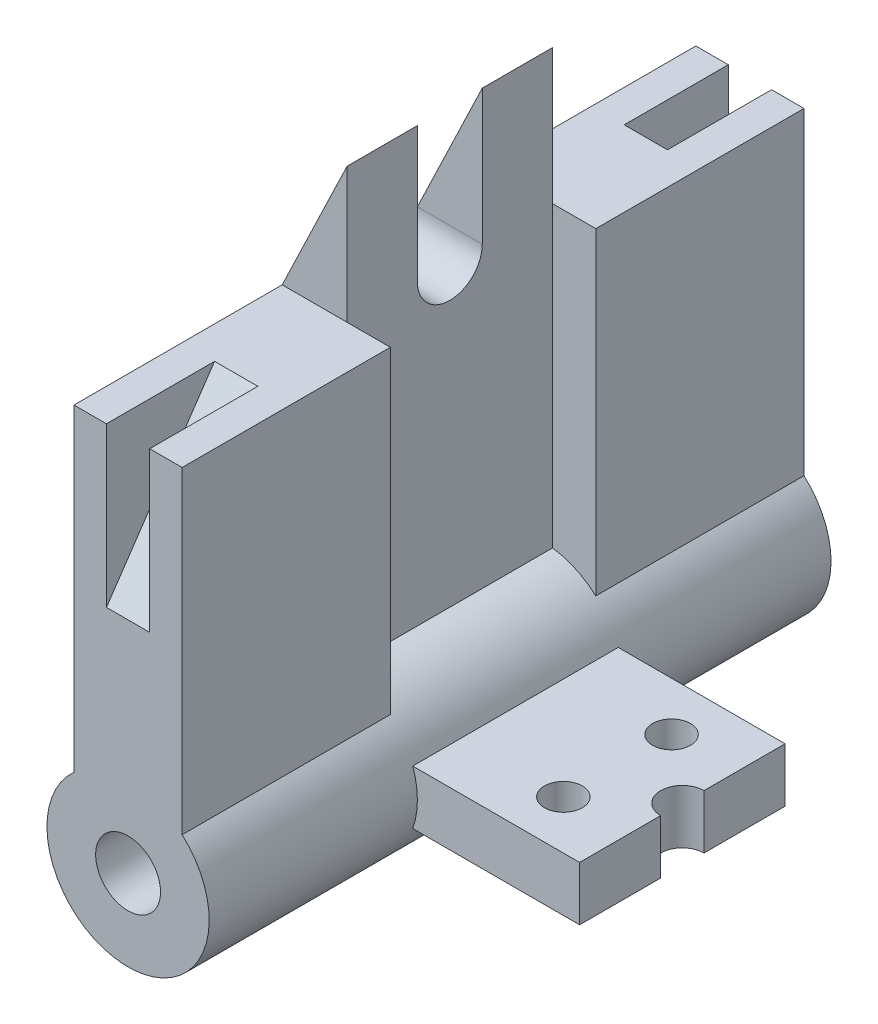
ISO-10303-21;
HEADER;
FILE_DESCRIPTION(('STEP AP214'),'2;1');
FILE_NAME('part.step','',(''),(''),'','','');
FILE_SCHEMA(('AUTOMOTIVE_DESIGN { 1 0 10303 214 1 1 1 1 }'));
ENDSEC;
DATA;
#1=APPLICATION_CONTEXT('core data for automotive mechanical design processes');
#2=APPLICATION_PROTOCOL_DEFINITION('international standard','automotive_design',2000,#1);
#3=PRODUCT_CONTEXT('',#1,'mechanical');
#4=PRODUCT('Part','Part','',(#3));
#5=PRODUCT_RELATED_PRODUCT_CATEGORY('part','',(#4));
#6=PRODUCT_DEFINITION_FORMATION('','',#4);
#7=PRODUCT_DEFINITION_CONTEXT('part definition',#1,'design');
#8=PRODUCT_DEFINITION('design','',#6,#7);
#9=PRODUCT_DEFINITION_SHAPE('','',#8);
#10=(LENGTH_UNIT() NAMED_UNIT(*) SI_UNIT(.MILLI.,.METRE.));
#11=(NAMED_UNIT(*) PLANE_ANGLE_UNIT() SI_UNIT($,.RADIAN.));
#12=(NAMED_UNIT(*) SI_UNIT($,.STERADIAN.) SOLID_ANGLE_UNIT());
#13=UNCERTAINTY_MEASURE_WITH_UNIT(LENGTH_MEASURE(1.E-05),#10,'distance_accuracy_value','');
#14=(GEOMETRIC_REPRESENTATION_CONTEXT(3) GLOBAL_UNCERTAINTY_ASSIGNED_CONTEXT((#13)) GLOBAL_UNIT_ASSIGNED_CONTEXT((#10,
#11,#12)) REPRESENTATION_CONTEXT('',''));
#15=CARTESIAN_POINT('',(0.,0.,0.));
#16=DIRECTION('',(0.,0.,1.));
#17=DIRECTION('',(1.,0.,0.));
#18=AXIS2_PLACEMENT_3D('',#15,#16,#17);
#19=CARTESIAN_POINT('',(-30.,5.,57.5));
#20=DIRECTION('',(0.,0.,1.));
#21=DIRECTION('',(1.,0.,0.));
#22=AXIS2_PLACEMENT_3D('',#19,#20,#21);
#23=PLANE('',#22);
#24=CARTESIAN_POINT('',(-30.,5.,57.5));
#25=DIRECTION('',(0.,0.,1.));
#26=DIRECTION('',(1.,0.,0.));
#27=AXIS2_PLACEMENT_3D('',#24,#25,#26);
#28=CIRCLE('',#27,6.);
#29=CARTESIAN_POINT('',(-24.,5.,57.5));
#30=VERTEX_POINT('',#29);
#31=EDGE_CURVE('E254',#30,#30,#28,.T.);
#32=ORIENTED_EDGE('',*,*,#31,.F.);
#33=EDGE_LOOP('',(#32));
#34=FACE_BOUND('',#33,.T.);
#35=DIRECTION('',(1.,0.,0.));
#36=VECTOR('',#35,1.);
#37=CARTESIAN_POINT('',(-34.,45.5901699437495,57.5));
#38=LINE('',#37,#36);
#39=CARTESIAN_POINT('',(-34.,45.5901699437495,57.5));
#40=VERTEX_POINT('',#39);
#41=CARTESIAN_POINT('',(-26.,45.5901699437495,57.5));
#42=VERTEX_POINT('',#41);
#43=EDGE_CURVE('E781',#40,#42,#38,.T.);
#44=ORIENTED_EDGE('',*,*,#43,.F.);
#45=DIRECTION('',(0.,-1.,0.));
#46=VECTOR('',#45,1.);
#47=CARTESIAN_POINT('',(-34.,75.,57.5));
#48=LINE('',#47,#46);
#49=CARTESIAN_POINT('',(-34.,75.,57.5));
#50=VERTEX_POINT('',#49);
#51=EDGE_CURVE('E779',#50,#40,#48,.T.);
#52=ORIENTED_EDGE('',*,*,#51,.F.);
#53=DIRECTION('',(-1.,0.,0.));
#54=VECTOR('',#53,1.);
#55=CARTESIAN_POINT('',(-20.,75.,57.5));
#56=LINE('',#55,#54);
#57=CARTESIAN_POINT('',(-40.,75.,57.5));
#58=VERTEX_POINT('',#57);
#59=EDGE_CURVE('E844',#50,#58,#56,.T.);
#60=ORIENTED_EDGE('',*,*,#59,.T.);
#61=DIRECTION('',(0.,1.,0.));
#62=VECTOR('',#61,1.);
#63=CARTESIAN_POINT('',(-40.,0.,57.5));
#64=LINE('',#63,#62);
#65=CARTESIAN_POINT('',(-40.,16.180339887499,57.5));
#66=VERTEX_POINT('',#65);
#67=EDGE_CURVE('E839',#66,#58,#64,.T.);
#68=ORIENTED_EDGE('',*,*,#67,.F.);
#69=CARTESIAN_POINT('',(-30.,5.,57.5));
#70=DIRECTION('',(0.,0.,1.));
#71=DIRECTION('',(1.,0.,0.));
#72=AXIS2_PLACEMENT_3D('',#69,#70,#71);
#73=CIRCLE('',#72,15.);
#74=CARTESIAN_POINT('',(-20.,16.180339887499,57.5));
#75=VERTEX_POINT('',#74);
#76=EDGE_CURVE('E257',#66,#75,#73,.T.);
#77=ORIENTED_EDGE('',*,*,#76,.T.);
#78=DIRECTION('',(0.,1.,0.));
#79=VECTOR('',#78,1.);
#80=CARTESIAN_POINT('',(-20.,0.,57.5));
#81=LINE('',#80,#79);
#82=CARTESIAN_POINT('',(-20.,75.,57.5));
#83=VERTEX_POINT('',#82);
#84=EDGE_CURVE('E842',#75,#83,#81,.T.);
#85=ORIENTED_EDGE('',*,*,#84,.T.);
#86=CARTESIAN_POINT('',(-26.,75.,57.5));
#87=VERTEX_POINT('',#86);
#88=EDGE_CURVE('E849',#83,#87,#56,.T.);
#89=ORIENTED_EDGE('',*,*,#88,.T.);
#90=DIRECTION('',(0.,-1.,0.));
#91=VECTOR('',#90,1.);
#92=CARTESIAN_POINT('',(-26.,75.,57.5));
#93=LINE('',#92,#91);
#94=EDGE_CURVE('E68',#87,#42,#93,.T.);
#95=ORIENTED_EDGE('',*,*,#94,.T.);
#96=EDGE_LOOP('',(#44,#52,#60,#68,#77,#85,#89,#95));
#97=FACE_BOUND('',#96,.T.);
#98=ADVANCED_FACE('F50',(#34,#97),#23,.T.);
#99=CARTESIAN_POINT('',(-20.,75.,0.));
#100=DIRECTION('',(0.,1.,0.));
#101=DIRECTION('',(0.,0.,1.));
#102=AXIS2_PLACEMENT_3D('',#99,#100,#101);
#103=PLANE('',#102);
#104=ORIENTED_EDGE('',*,*,#59,.F.);
#105=DIRECTION('',(0.,0.,1.));
#106=VECTOR('',#105,1.);
#107=CARTESIAN_POINT('',(-34.,75.,37.5));
#108=LINE('',#107,#106);
#109=CARTESIAN_POINT('',(-34.,75.,37.5));
#110=VERTEX_POINT('',#109);
#111=EDGE_CURVE('E777',#110,#50,#108,.T.);
#112=ORIENTED_EDGE('',*,*,#111,.F.);
#113=DIRECTION('',(1.,0.,0.));
#114=VECTOR('',#113,1.);
#115=CARTESIAN_POINT('',(-34.,75.,37.5));
#116=LINE('',#115,#114);
#117=CARTESIAN_POINT('',(-26.,75.,37.5));
#118=VERTEX_POINT('',#117);
#119=EDGE_CURVE('E764',#110,#118,#116,.T.);
#120=ORIENTED_EDGE('',*,*,#119,.T.);
#121=DIRECTION('',(0.,0.,1.));
#122=VECTOR('',#121,1.);
#123=CARTESIAN_POINT('',(-26.,75.,37.5));
#124=LINE('',#123,#122);
#125=EDGE_CURVE('E783',#118,#87,#124,.T.);
#126=ORIENTED_EDGE('',*,*,#125,.T.);
#127=ORIENTED_EDGE('',*,*,#88,.F.);
#128=DIRECTION('',(0.,0.,-1.));
#129=VECTOR('',#128,1.);
#130=CARTESIAN_POINT('',(-20.,75.,0.));
#131=LINE('',#130,#129);
#132=CARTESIAN_POINT('',(-20.,75.,19.));
#133=VERTEX_POINT('',#132);
#134=EDGE_CURVE('E840',#83,#133,#131,.T.);
#135=ORIENTED_EDGE('',*,*,#134,.T.);
#136=DIRECTION('',(-1.,0.,0.));
#137=VECTOR('',#136,1.);
#138=CARTESIAN_POINT('',(-20.,75.,19.));
#139=LINE('',#138,#137);
#140=CARTESIAN_POINT('',(-28.,75.,19.));
#141=VERTEX_POINT('',#140);
#142=EDGE_CURVE('E854',#133,#141,#139,.T.);
#143=ORIENTED_EDGE('',*,*,#142,.T.);
#144=DIRECTION('',(1.,0.,0.));
#145=VECTOR('',#144,1.);
#146=CARTESIAN_POINT('',(-20.,75.,19.));
#147=LINE('',#146,#145);
#148=CARTESIAN_POINT('',(-40.,75.,19.));
#149=VERTEX_POINT('',#148);
#150=EDGE_CURVE('E822',#149,#141,#147,.T.);
#151=ORIENTED_EDGE('',*,*,#150,.F.);
#152=DIRECTION('',(0.,0.,-1.));
#153=VECTOR('',#152,1.);
#154=CARTESIAN_POINT('',(-40.,75.,0.));
#155=LINE('',#154,#153);
#156=EDGE_CURVE('E833',#58,#149,#155,.T.);
#157=ORIENTED_EDGE('',*,*,#156,.F.);
#158=EDGE_LOOP('',(#104,#112,#120,#126,#127,#135,#143,#151,#157));
#159=FACE_BOUND('',#158,.T.);
#160=ADVANCED_FACE('F361',(#159),#103,.T.);
#161=CARTESIAN_POINT('',(-30.,5.,-57.5));
#162=DIRECTION('',(0.,0.,1.));
#163=DIRECTION('',(1.,0.,0.));
#164=AXIS2_PLACEMENT_3D('',#161,#162,#163);
#165=CYLINDRICAL_SURFACE('',#164,15.);
#166=DIRECTION('',(0.,0.,1.));
#167=VECTOR('',#166,1.);
#168=CARTESIAN_POINT('',(-15.857864376269,0.,-57.5));
#169=LINE('',#168,#167);
#170=CARTESIAN_POINT('',(-15.857864376269,0.,19.));
#171=VERTEX_POINT('',#170);
#172=CARTESIAN_POINT('',(-15.857864376269,0.,-19.));
#173=VERTEX_POINT('',#172);
#174=EDGE_CURVE('E268',#171,#173,#169,.F.);
#175=ORIENTED_EDGE('',*,*,#174,.F.);
#176=CARTESIAN_POINT('',(-30.,5.,19.));
#177=DIRECTION('',(0.,0.,1.));
#178=DIRECTION('',(1.,0.,0.));
#179=AXIS2_PLACEMENT_3D('',#176,#177,#178);
#180=CIRCLE('',#179,15.);
#181=CARTESIAN_POINT('',(-15.857864376269,10.,19.));
#182=VERTEX_POINT('',#181);
#183=EDGE_CURVE('E258',#171,#182,#180,.T.);
#184=ORIENTED_EDGE('',*,*,#183,.T.);
#185=DIRECTION('',(0.,0.,1.));
#186=VECTOR('',#185,1.);
#187=CARTESIAN_POINT('',(-15.857864376269,10.,-57.5));
#188=LINE('',#187,#186);
#189=CARTESIAN_POINT('',(-15.857864376269,10.,-19.));
#190=VERTEX_POINT('',#189);
#191=EDGE_CURVE('E275',#182,#190,#188,.F.);
#192=ORIENTED_EDGE('',*,*,#191,.T.);
#193=CARTESIAN_POINT('',(-30.,5.,-19.));
#194=DIRECTION('',(0.,0.,1.));
#195=DIRECTION('',(1.,0.,0.));
#196=AXIS2_PLACEMENT_3D('',#193,#194,#195);
#197=CIRCLE('',#196,15.);
#198=EDGE_CURVE('E264',#173,#190,#197,.T.);
#199=ORIENTED_EDGE('',*,*,#198,.F.);
#200=EDGE_LOOP('',(#175,#184,#192,#199));
#201=FACE_BOUND('',#200,.T.);
#202=CARTESIAN_POINT('',(-30.,5.,-19.));
#203=DIRECTION('',(0.,0.,1.));
#204=DIRECTION('',(1.,0.,0.));
#205=AXIS2_PLACEMENT_3D('',#202,#203,#204);
#206=CIRCLE('',#205,15.);
#207=CARTESIAN_POINT('',(-28.,19.8660687473185,-19.));
#208=VERTEX_POINT('',#207);
#209=CARTESIAN_POINT('',(-20.,16.180339887499,-19.));
#210=VERTEX_POINT('',#209);
#211=EDGE_CURVE('E241',#208,#210,#206,.F.);
#212=ORIENTED_EDGE('',*,*,#211,.F.);
#213=DIRECTION('',(0.,0.,1.));
#214=VECTOR('',#213,1.);
#215=CARTESIAN_POINT('',(-28.,19.8660687473185,-57.5));
#216=LINE('',#215,#214);
#217=CARTESIAN_POINT('',(-28.,19.8660687473185,19.));
#218=VERTEX_POINT('',#217);
#219=EDGE_CURVE('E827',#208,#218,#216,.T.);
#220=ORIENTED_EDGE('',*,*,#219,.T.);
#221=CARTESIAN_POINT('',(-30.,5.,19.));
#222=DIRECTION('',(0.,0.,1.));
#223=DIRECTION('',(1.,0.,0.));
#224=AXIS2_PLACEMENT_3D('',#221,#222,#223);
#225=CIRCLE('',#224,15.);
#226=CARTESIAN_POINT('',(-20.,16.180339887499,19.));
#227=VERTEX_POINT('',#226);
#228=EDGE_CURVE('E860',#218,#227,#225,.F.);
#229=ORIENTED_EDGE('',*,*,#228,.T.);
#230=DIRECTION('',(0.,0.,1.));
#231=VECTOR('',#230,1.);
#232=CARTESIAN_POINT('',(-20.,16.180339887499,-57.5));
#233=LINE('',#232,#231);
#234=EDGE_CURVE('E853',#75,#227,#233,.F.);
#235=ORIENTED_EDGE('',*,*,#234,.F.);
#236=ORIENTED_EDGE('',*,*,#76,.F.);
#237=DIRECTION('',(0.,0.,1.));
#238=VECTOR('',#237,1.);
#239=CARTESIAN_POINT('',(-40.,16.1803398874989,-57.5));
#240=LINE('',#239,#238);
#241=CARTESIAN_POINT('',(-40.,16.1803398874989,-57.5));
#242=VERTEX_POINT('',#241);
#243=EDGE_CURVE('E247',#66,#242,#240,.F.);
#244=ORIENTED_EDGE('',*,*,#243,.T.);
#245=CARTESIAN_POINT('',(-30.,5.,-57.5));
#246=DIRECTION('',(0.,0.,1.));
#247=DIRECTION('',(1.,0.,0.));
#248=AXIS2_PLACEMENT_3D('',#245,#246,#247);
#249=CIRCLE('',#248,15.);
#250=CARTESIAN_POINT('',(-20.,16.180339887499,-57.5));
#251=VERTEX_POINT('',#250);
#252=EDGE_CURVE('E269',#242,#251,#249,.T.);
#253=ORIENTED_EDGE('',*,*,#252,.T.);
#254=DIRECTION('',(0.,0.,1.));
#255=VECTOR('',#254,1.);
#256=CARTESIAN_POINT('',(-20.,16.180339887499,-57.5));
#257=LINE('',#256,#255);
#258=EDGE_CURVE('E252',#210,#251,#257,.F.);
#259=ORIENTED_EDGE('',*,*,#258,.F.);
#260=EDGE_LOOP('',(#212,#220,#229,#235,#236,#244,#253,#259));
#261=FACE_BOUND('',#260,.T.);
#262=ADVANCED_FACE('F344',(#201,#261),#165,.T.);
#263=CARTESIAN_POINT('',(-20.,0.,-19.));
#264=DIRECTION('',(0.,0.,1.));
#265=DIRECTION('',(1.,0.,0.));
#266=AXIS2_PLACEMENT_3D('',#263,#264,#265);
#267=PLANE('',#266);
#268=DIRECTION('',(-1.,0.,0.));
#269=VECTOR('',#268,1.);
#270=CARTESIAN_POINT('',(-20.,75.,-19.));
#271=LINE('',#270,#269);
#272=CARTESIAN_POINT('',(-20.,75.,-19.));
#273=VERTEX_POINT('',#272);
#274=CARTESIAN_POINT('',(-28.,75.,-19.));
#275=VERTEX_POINT('',#274);
#276=EDGE_CURVE('E238',#273,#275,#271,.T.);
#277=ORIENTED_EDGE('',*,*,#276,.T.);
#278=DIRECTION('',(0.,-1.,0.));
#279=VECTOR('',#278,1.);
#280=CARTESIAN_POINT('',(-28.,16.1803398874989,-19.));
#281=LINE('',#280,#279);
#282=EDGE_CURVE('E809',#275,#208,#281,.T.);
#283=ORIENTED_EDGE('',*,*,#282,.T.);
#284=ORIENTED_EDGE('',*,*,#211,.T.);
#285=DIRECTION('',(0.,1.,0.));
#286=VECTOR('',#285,1.);
#287=CARTESIAN_POINT('',(-20.,0.,-19.));
#288=LINE('',#287,#286);
#289=EDGE_CURVE('E859',#210,#273,#288,.T.);
#290=ORIENTED_EDGE('',*,*,#289,.T.);
#291=EDGE_LOOP('',(#277,#283,#284,#290));
#292=FACE_BOUND('',#291,.T.);
#293=ADVANCED_FACE('F376',(#292),#267,.T.);
#294=CARTESIAN_POINT('',(-20.,0.,19.));
#295=DIRECTION('',(0.,0.,1.));
#296=DIRECTION('',(1.,0.,0.));
#297=AXIS2_PLACEMENT_3D('',#294,#295,#296);
#298=PLANE('',#297);
#299=DIRECTION('',(0.,1.,0.));
#300=VECTOR('',#299,1.);
#301=CARTESIAN_POINT('',(-28.,16.1803398874989,19.));
#302=LINE('',#301,#300);
#303=EDGE_CURVE('E808',#218,#141,#302,.T.);
#304=ORIENTED_EDGE('',*,*,#303,.T.);
#305=ORIENTED_EDGE('',*,*,#142,.F.);
#306=DIRECTION('',(0.,1.,0.));
#307=VECTOR('',#306,1.);
#308=CARTESIAN_POINT('',(-20.,0.,19.));
#309=LINE('',#308,#307);
#310=EDGE_CURVE('E834',#227,#133,#309,.T.);
#311=ORIENTED_EDGE('',*,*,#310,.F.);
#312=ORIENTED_EDGE('',*,*,#228,.F.);
#313=EDGE_LOOP('',(#304,#305,#311,#312));
#314=FACE_BOUND('',#313,.T.);
#315=ADVANCED_FACE('F379',(#314),#298,.F.);
#316=CARTESIAN_POINT('',(-30.,5.,-57.5));
#317=DIRECTION('',(0.,0.,1.));
#318=DIRECTION('',(1.,0.,0.));
#319=AXIS2_PLACEMENT_3D('',#316,#317,#318);
#320=CYLINDRICAL_SURFACE('',#319,6.);
#321=CARTESIAN_POINT('',(-30.,5.,-57.5));
#322=DIRECTION('',(0.,0.,1.));
#323=DIRECTION('',(1.,0.,0.));
#324=AXIS2_PLACEMENT_3D('',#321,#322,#323);
#325=CIRCLE('',#324,6.);
#326=CARTESIAN_POINT('',(-24.,5.,-57.5));
#327=VERTEX_POINT('',#326);
#328=EDGE_CURVE('E256',#327,#327,#325,.T.);
#329=ORIENTED_EDGE('',*,*,#328,.F.);
#330=EDGE_LOOP('',(#329));
#331=FACE_BOUND('',#330,.T.);
#332=ORIENTED_EDGE('',*,*,#31,.T.);
#333=EDGE_LOOP('',(#332));
#334=FACE_BOUND('',#333,.T.);
#335=ADVANCED_FACE('F377',(#331,#334),#320,.F.);
#336=CARTESIAN_POINT('',(15.,10.,0.));
#337=DIRECTION('',(0.,1.,0.));
#338=DIRECTION('',(0.,0.,1.));
#339=AXIS2_PLACEMENT_3D('',#336,#337,#338);
#340=PLANE('',#339);
#341=ORIENTED_EDGE('',*,*,#191,.F.);
#342=DIRECTION('',(1.,0.,0.));
#343=VECTOR('',#342,1.);
#344=CARTESIAN_POINT('',(-15.,10.,19.));
#345=LINE('',#344,#343);
#346=CARTESIAN_POINT('',(15.,10.,19.));
#347=VERTEX_POINT('',#346);
#348=EDGE_CURVE('E286',#182,#347,#345,.T.);
#349=ORIENTED_EDGE('',*,*,#348,.T.);
#350=DIRECTION('',(0.,0.,-1.));
#351=VECTOR('',#350,1.);
#352=CARTESIAN_POINT('',(15.,10.,4.));
#353=LINE('',#352,#351);
#354=CARTESIAN_POINT('',(15.,10.,4.));
#355=VERTEX_POINT('',#354);
#356=EDGE_CURVE('E288',#347,#355,#353,.T.);
#357=ORIENTED_EDGE('',*,*,#356,.T.);
#358=CARTESIAN_POINT('',(15.,10.,0.));
#359=DIRECTION('',(0.,-1.,0.));
#360=DIRECTION('',(0.,0.,1.));
#361=AXIS2_PLACEMENT_3D('',#358,#359,#360);
#362=CIRCLE('',#361,4.);
#363=CARTESIAN_POINT('',(15.,10.,-4.));
#364=VERTEX_POINT('',#363);
#365=EDGE_CURVE('E292',#355,#364,#362,.T.);
#366=ORIENTED_EDGE('',*,*,#365,.T.);
#367=DIRECTION('',(0.,0.,-1.));
#368=VECTOR('',#367,1.);
#369=CARTESIAN_POINT('',(15.,10.,-19.));
#370=LINE('',#369,#368);
#371=CARTESIAN_POINT('',(15.,10.,-19.));
#372=VERTEX_POINT('',#371);
#373=EDGE_CURVE('E295',#364,#372,#370,.T.);
#374=ORIENTED_EDGE('',*,*,#373,.T.);
#375=DIRECTION('',(-1.,0.,0.));
#376=VECTOR('',#375,1.);
#377=CARTESIAN_POINT('',(-15.,10.,-19.));
#378=LINE('',#377,#376);
#379=EDGE_CURVE('E298',#372,#190,#378,.T.);
#380=ORIENTED_EDGE('',*,*,#379,.T.);
#381=EDGE_LOOP('',(#341,#349,#357,#366,#374,#380));
#382=FACE_BOUND('',#381,.T.);
#383=CARTESIAN_POINT('',(3.,10.,-10.));
#384=DIRECTION('',(0.,1.,0.));
#385=DIRECTION('',(0.,0.,1.));
#386=AXIS2_PLACEMENT_3D('',#383,#384,#385);
#387=CIRCLE('',#386,3.5);
#388=CARTESIAN_POINT('',(3.,10.,-6.5));
#389=VERTEX_POINT('',#388);
#390=EDGE_CURVE('E282',#389,#389,#387,.T.);
#391=ORIENTED_EDGE('',*,*,#390,.F.);
#392=EDGE_LOOP('',(#391));
#393=FACE_BOUND('',#392,.T.);
#394=CARTESIAN_POINT('',(3.,10.,10.));
#395=DIRECTION('',(0.,1.,0.));
#396=DIRECTION('',(0.,0.,1.));
#397=AXIS2_PLACEMENT_3D('',#394,#395,#396);
#398=CIRCLE('',#397,3.5);
#399=CARTESIAN_POINT('',(3.,10.,13.5));
#400=VERTEX_POINT('',#399);
#401=EDGE_CURVE('E273',#400,#400,#398,.T.);
#402=ORIENTED_EDGE('',*,*,#401,.F.);
#403=EDGE_LOOP('',(#402));
#404=FACE_BOUND('',#403,.T.);
#405=ADVANCED_FACE('F329',(#382,#393,#404),#340,.T.);
#406=CARTESIAN_POINT('',(15.,0.,0.));
#407=DIRECTION('',(0.,1.,0.));
#408=DIRECTION('',(0.,0.,1.));
#409=AXIS2_PLACEMENT_3D('',#406,#407,#408);
#410=PLANE('',#409);
#411=DIRECTION('',(1.,0.,0.));
#412=VECTOR('',#411,1.);
#413=CARTESIAN_POINT('',(-15.,0.,19.));
#414=LINE('',#413,#412);
#415=CARTESIAN_POINT('',(15.,0.,19.));
#416=VERTEX_POINT('',#415);
#417=EDGE_CURVE('E281',#171,#416,#414,.T.);
#418=ORIENTED_EDGE('',*,*,#417,.F.);
#419=ORIENTED_EDGE('',*,*,#174,.T.);
#420=DIRECTION('',(-1.,0.,0.));
#421=VECTOR('',#420,1.);
#422=CARTESIAN_POINT('',(-15.,0.,-19.));
#423=LINE('',#422,#421);
#424=CARTESIAN_POINT('',(15.,0.,-19.));
#425=VERTEX_POINT('',#424);
#426=EDGE_CURVE('E287',#425,#173,#423,.T.);
#427=ORIENTED_EDGE('',*,*,#426,.F.);
#428=DIRECTION('',(0.,0.,-1.));
#429=VECTOR('',#428,1.);
#430=CARTESIAN_POINT('',(15.,0.,-19.));
#431=LINE('',#430,#429);
#432=CARTESIAN_POINT('',(15.,0.,-4.));
#433=VERTEX_POINT('',#432);
#434=EDGE_CURVE('E304',#433,#425,#431,.T.);
#435=ORIENTED_EDGE('',*,*,#434,.F.);
#436=CARTESIAN_POINT('',(15.,0.,0.));
#437=DIRECTION('',(0.,-1.,0.));
#438=DIRECTION('',(0.,0.,1.));
#439=AXIS2_PLACEMENT_3D('',#436,#437,#438);
#440=CIRCLE('',#439,4.);
#441=CARTESIAN_POINT('',(15.,0.,4.));
#442=VERTEX_POINT('',#441);
#443=EDGE_CURVE('E303',#442,#433,#440,.T.);
#444=ORIENTED_EDGE('',*,*,#443,.F.);
#445=DIRECTION('',(0.,0.,-1.));
#446=VECTOR('',#445,1.);
#447=CARTESIAN_POINT('',(15.,0.,4.));
#448=LINE('',#447,#446);
#449=EDGE_CURVE('E301',#416,#442,#448,.T.);
#450=ORIENTED_EDGE('',*,*,#449,.F.);
#451=EDGE_LOOP('',(#418,#419,#427,#435,#444,#450));
#452=FACE_BOUND('',#451,.T.);
#453=CARTESIAN_POINT('',(3.,0.,-10.));
#454=DIRECTION('',(0.,1.,0.));
#455=DIRECTION('',(0.,0.,1.));
#456=AXIS2_PLACEMENT_3D('',#453,#454,#455);
#457=CIRCLE('',#456,3.5);
#458=CARTESIAN_POINT('',(3.,0.,-6.5));
#459=VERTEX_POINT('',#458);
#460=EDGE_CURVE('E279',#459,#459,#457,.T.);
#461=ORIENTED_EDGE('',*,*,#460,.T.);
#462=EDGE_LOOP('',(#461));
#463=FACE_BOUND('',#462,.T.);
#464=CARTESIAN_POINT('',(3.,0.,10.));
#465=DIRECTION('',(0.,1.,0.));
#466=DIRECTION('',(0.,0.,1.));
#467=AXIS2_PLACEMENT_3D('',#464,#465,#466);
#468=CIRCLE('',#467,3.5);
#469=CARTESIAN_POINT('',(3.,0.,13.5));
#470=VERTEX_POINT('',#469);
#471=EDGE_CURVE('E274',#470,#470,#468,.T.);
#472=ORIENTED_EDGE('',*,*,#471,.T.);
#473=EDGE_LOOP('',(#472));
#474=FACE_BOUND('',#473,.T.);
#475=ADVANCED_FACE('F339',(#452,#463,#474),#410,.F.);
#476=CARTESIAN_POINT('',(-15.,10.,19.));
#477=DIRECTION('',(0.,0.,-1.));
#478=DIRECTION('',(-1.,0.,0.));
#479=AXIS2_PLACEMENT_3D('',#476,#477,#478);
#480=PLANE('',#479);
#481=ORIENTED_EDGE('',*,*,#183,.F.);
#482=ORIENTED_EDGE('',*,*,#417,.T.);
#483=DIRECTION('',(0.,-1.,0.));
#484=VECTOR('',#483,1.);
#485=CARTESIAN_POINT('',(15.,10.,19.));
#486=LINE('',#485,#484);
#487=EDGE_CURVE('E320',#347,#416,#486,.T.);
#488=ORIENTED_EDGE('',*,*,#487,.F.);
#489=ORIENTED_EDGE('',*,*,#348,.F.);
#490=EDGE_LOOP('',(#481,#482,#488,#489));
#491=FACE_BOUND('',#490,.T.);
#492=ADVANCED_FACE('F47',(#491),#480,.F.);
#493=CARTESIAN_POINT('',(15.,10.,4.));
#494=DIRECTION('',(-1.,0.,0.));
#495=DIRECTION('',(0.,0.,1.));
#496=AXIS2_PLACEMENT_3D('',#493,#494,#495);
#497=PLANE('',#496);
#498=ORIENTED_EDGE('',*,*,#449,.T.);
#499=DIRECTION('',(0.,-1.,0.));
#500=VECTOR('',#499,1.);
#501=CARTESIAN_POINT('',(15.,10.,4.));
#502=LINE('',#501,#500);
#503=EDGE_CURVE('E313',#355,#442,#502,.T.);
#504=ORIENTED_EDGE('',*,*,#503,.F.);
#505=ORIENTED_EDGE('',*,*,#356,.F.);
#506=ORIENTED_EDGE('',*,*,#487,.T.);
#507=EDGE_LOOP('',(#498,#504,#505,#506));
#508=FACE_BOUND('',#507,.T.);
#509=ADVANCED_FACE('F348',(#508),#497,.F.);
#510=CARTESIAN_POINT('',(15.,10.,0.));
#511=DIRECTION('',(0.,-1.,0.));
#512=DIRECTION('',(0.,0.,-1.));
#513=AXIS2_PLACEMENT_3D('',#510,#511,#512);
#514=CYLINDRICAL_SURFACE('',#513,4.);
#515=ORIENTED_EDGE('',*,*,#443,.T.);
#516=DIRECTION('',(0.,-1.,0.));
#517=VECTOR('',#516,1.);
#518=CARTESIAN_POINT('',(15.,10.,-4.));
#519=LINE('',#518,#517);
#520=EDGE_CURVE('E311',#364,#433,#519,.T.);
#521=ORIENTED_EDGE('',*,*,#520,.F.);
#522=ORIENTED_EDGE('',*,*,#365,.F.);
#523=ORIENTED_EDGE('',*,*,#503,.T.);
#524=EDGE_LOOP('',(#515,#521,#522,#523));
#525=FACE_BOUND('',#524,.T.);
#526=ADVANCED_FACE('F351',(#525),#514,.F.);
#527=CARTESIAN_POINT('',(15.,10.,-19.));
#528=DIRECTION('',(-1.,0.,0.));
#529=DIRECTION('',(0.,0.,1.));
#530=AXIS2_PLACEMENT_3D('',#527,#528,#529);
#531=PLANE('',#530);
#532=ORIENTED_EDGE('',*,*,#434,.T.);
#533=DIRECTION('',(0.,-1.,0.));
#534=VECTOR('',#533,1.);
#535=CARTESIAN_POINT('',(15.,10.,-19.));
#536=LINE('',#535,#534);
#537=EDGE_CURVE('E299',#372,#425,#536,.T.);
#538=ORIENTED_EDGE('',*,*,#537,.F.);
#539=ORIENTED_EDGE('',*,*,#373,.F.);
#540=ORIENTED_EDGE('',*,*,#520,.T.);
#541=EDGE_LOOP('',(#532,#538,#539,#540));
#542=FACE_BOUND('',#541,.T.);
#543=ADVANCED_FACE('F332',(#542),#531,.F.);
#544=CARTESIAN_POINT('',(-15.,10.,-19.));
#545=DIRECTION('',(0.,0.,1.));
#546=DIRECTION('',(1.,0.,0.));
#547=AXIS2_PLACEMENT_3D('',#544,#545,#546);
#548=PLANE('',#547);
#549=ORIENTED_EDGE('',*,*,#426,.T.);
#550=ORIENTED_EDGE('',*,*,#198,.T.);
#551=ORIENTED_EDGE('',*,*,#379,.F.);
#552=ORIENTED_EDGE('',*,*,#537,.T.);
#553=EDGE_LOOP('',(#549,#550,#551,#552));
#554=FACE_BOUND('',#553,.T.);
#555=ADVANCED_FACE('F325',(#554),#548,.F.);
#556=CARTESIAN_POINT('',(3.,10.,-10.));
#557=DIRECTION('',(0.,-1.,0.));
#558=DIRECTION('',(0.,0.,-1.));
#559=AXIS2_PLACEMENT_3D('',#556,#557,#558);
#560=CYLINDRICAL_SURFACE('',#559,3.5);
#561=ORIENTED_EDGE('',*,*,#390,.T.);
#562=EDGE_LOOP('',(#561));
#563=FACE_BOUND('',#562,.T.);
#564=ORIENTED_EDGE('',*,*,#460,.F.);
#565=EDGE_LOOP('',(#564));
#566=FACE_BOUND('',#565,.T.);
#567=ADVANCED_FACE('F388',(#563,#566),#560,.F.);
#568=CARTESIAN_POINT('',(3.,10.,10.));
#569=DIRECTION('',(0.,-1.,0.));
#570=DIRECTION('',(0.,0.,-1.));
#571=AXIS2_PLACEMENT_3D('',#568,#569,#570);
#572=CYLINDRICAL_SURFACE('',#571,3.5);
#573=ORIENTED_EDGE('',*,*,#401,.T.);
#574=EDGE_LOOP('',(#573));
#575=FACE_BOUND('',#574,.T.);
#576=ORIENTED_EDGE('',*,*,#471,.F.);
#577=EDGE_LOOP('',(#576));
#578=FACE_BOUND('',#577,.T.);
#579=ADVANCED_FACE('F381',(#575,#578),#572,.F.);
#580=CARTESIAN_POINT('',(-30.,5.,-57.5));
#581=DIRECTION('',(0.,0.,1.));
#582=DIRECTION('',(1.,0.,0.));
#583=AXIS2_PLACEMENT_3D('',#580,#581,#582);
#584=PLANE('',#583);
#585=ORIENTED_EDGE('',*,*,#328,.T.);
#586=EDGE_LOOP('',(#585));
#587=FACE_BOUND('',#586,.T.);
#588=DIRECTION('',(-1.,0.,0.));
#589=VECTOR('',#588,1.);
#590=CARTESIAN_POINT('',(-20.,75.,-57.5));
#591=LINE('',#590,#589);
#592=CARTESIAN_POINT('',(-34.,75.,-57.5));
#593=VERTEX_POINT('',#592);
#594=CARTESIAN_POINT('',(-40.,75.,-57.5));
#595=VERTEX_POINT('',#594);
#596=EDGE_CURVE('E226',#593,#595,#591,.T.);
#597=ORIENTED_EDGE('',*,*,#596,.F.);
#598=DIRECTION('',(0.,1.,0.));
#599=VECTOR('',#598,1.);
#600=CARTESIAN_POINT('',(-34.,75.,-57.5));
#601=LINE('',#600,#599);
#602=CARTESIAN_POINT('',(-34.,45.5901699437495,-57.5));
#603=VERTEX_POINT('',#602);
#604=EDGE_CURVE('E213',#603,#593,#601,.T.);
#605=ORIENTED_EDGE('',*,*,#604,.F.);
#606=DIRECTION('',(1.,0.,0.));
#607=VECTOR('',#606,1.);
#608=CARTESIAN_POINT('',(-34.,45.5901699437495,-57.5));
#609=LINE('',#608,#607);
#610=CARTESIAN_POINT('',(-26.,45.5901699437495,-57.5));
#611=VERTEX_POINT('',#610);
#612=EDGE_CURVE('E770',#603,#611,#609,.T.);
#613=ORIENTED_EDGE('',*,*,#612,.T.);
#614=DIRECTION('',(0.,1.,0.));
#615=VECTOR('',#614,1.);
#616=CARTESIAN_POINT('',(-26.,75.,-57.5));
#617=LINE('',#616,#615);
#618=CARTESIAN_POINT('',(-26.,75.,-57.5));
#619=VERTEX_POINT('',#618);
#620=EDGE_CURVE('E765',#611,#619,#617,.T.);
#621=ORIENTED_EDGE('',*,*,#620,.T.);
#622=CARTESIAN_POINT('',(-20.,75.,-57.5));
#623=VERTEX_POINT('',#622);
#624=EDGE_CURVE('E240',#623,#619,#591,.T.);
#625=ORIENTED_EDGE('',*,*,#624,.F.);
#626=DIRECTION('',(0.,1.,0.));
#627=VECTOR('',#626,1.);
#628=CARTESIAN_POINT('',(-20.,0.,-57.5));
#629=LINE('',#628,#627);
#630=EDGE_CURVE('E862',#251,#623,#629,.T.);
#631=ORIENTED_EDGE('',*,*,#630,.F.);
#632=ORIENTED_EDGE('',*,*,#252,.F.);
#633=DIRECTION('',(0.,1.,0.));
#634=VECTOR('',#633,1.);
#635=CARTESIAN_POINT('',(-40.,0.,-57.5));
#636=LINE('',#635,#634);
#637=EDGE_CURVE('E232',#242,#595,#636,.T.);
#638=ORIENTED_EDGE('',*,*,#637,.T.);
#639=EDGE_LOOP('',(#597,#605,#613,#621,#625,#631,#632,#638));
#640=FACE_BOUND('',#639,.T.);
#641=ADVANCED_FACE('F231',(#587,#640),#584,.F.);
#642=CARTESIAN_POINT('',(-20.,75.,0.));
#643=DIRECTION('',(0.,-1.,0.));
#644=DIRECTION('',(0.,0.,-1.));
#645=AXIS2_PLACEMENT_3D('',#642,#643,#644);
#646=PLANE('',#645);
#647=DIRECTION('',(1.,0.,0.));
#648=VECTOR('',#647,1.);
#649=CARTESIAN_POINT('',(-34.,75.,-38.25));
#650=LINE('',#649,#648);
#651=CARTESIAN_POINT('',(-34.,75.,-38.25));
#652=VERTEX_POINT('',#651);
#653=CARTESIAN_POINT('',(-26.,75.,-38.25));
#654=VERTEX_POINT('',#653);
#655=EDGE_CURVE('E233',#652,#654,#650,.T.);
#656=ORIENTED_EDGE('',*,*,#655,.F.);
#657=DIRECTION('',(0.,0.,1.));
#658=VECTOR('',#657,1.);
#659=CARTESIAN_POINT('',(-34.,75.,-57.5));
#660=LINE('',#659,#658);
#661=EDGE_CURVE('E219',#593,#652,#660,.T.);
#662=ORIENTED_EDGE('',*,*,#661,.F.);
#663=ORIENTED_EDGE('',*,*,#596,.T.);
#664=DIRECTION('',(0.,0.,1.));
#665=VECTOR('',#664,1.);
#666=CARTESIAN_POINT('',(-40.,75.,0.));
#667=LINE('',#666,#665);
#668=CARTESIAN_POINT('',(-40.,75.,-19.));
#669=VERTEX_POINT('',#668);
#670=EDGE_CURVE('E865',#595,#669,#667,.T.);
#671=ORIENTED_EDGE('',*,*,#670,.T.);
#672=DIRECTION('',(1.,0.,0.));
#673=VECTOR('',#672,1.);
#674=CARTESIAN_POINT('',(-20.,75.,-19.));
#675=LINE('',#674,#673);
#676=EDGE_CURVE('E831',#669,#275,#675,.T.);
#677=ORIENTED_EDGE('',*,*,#676,.T.);
#678=ORIENTED_EDGE('',*,*,#276,.F.);
#679=DIRECTION('',(0.,0.,1.));
#680=VECTOR('',#679,1.);
#681=CARTESIAN_POINT('',(-20.,75.,0.));
#682=LINE('',#681,#680);
#683=EDGE_CURVE('E243',#623,#273,#682,.T.);
#684=ORIENTED_EDGE('',*,*,#683,.F.);
#685=ORIENTED_EDGE('',*,*,#624,.T.);
#686=DIRECTION('',(0.,0.,1.));
#687=VECTOR('',#686,1.);
#688=CARTESIAN_POINT('',(-26.,75.,-57.5));
#689=LINE('',#688,#687);
#690=EDGE_CURVE('E763',#619,#654,#689,.T.);
#691=ORIENTED_EDGE('',*,*,#690,.T.);
#692=EDGE_LOOP('',(#656,#662,#663,#671,#677,#678,#684,#685,#691));
#693=FACE_BOUND('',#692,.T.);
#694=ADVANCED_FACE('F227',(#693),#646,.F.);
#695=CARTESIAN_POINT('',(-20.,0.,0.));
#696=DIRECTION('',(1.,0.,0.));
#697=DIRECTION('',(0.,0.,-1.));
#698=AXIS2_PLACEMENT_3D('',#695,#696,#697);
#699=PLANE('',#698);
#700=ORIENTED_EDGE('',*,*,#289,.F.);
#701=ORIENTED_EDGE('',*,*,#258,.T.);
#702=ORIENTED_EDGE('',*,*,#630,.T.);
#703=ORIENTED_EDGE('',*,*,#683,.T.);
#704=EDGE_LOOP('',(#700,#701,#702,#703));
#705=FACE_BOUND('',#704,.T.);
#706=ADVANCED_FACE('F417',(#705),#699,.T.);
#707=CARTESIAN_POINT('',(-40.,0.,0.));
#708=DIRECTION('',(1.,0.,0.));
#709=DIRECTION('',(0.,0.,-1.));
#710=AXIS2_PLACEMENT_3D('',#707,#708,#709);
#711=PLANE('',#710);
#712=ORIENTED_EDGE('',*,*,#156,.T.);
#713=DIRECTION('',(0.,0.,1.));
#714=VECTOR('',#713,1.);
#715=CARTESIAN_POINT('',(-40.,75.,-31.));
#716=LINE('',#715,#714);
#717=CARTESIAN_POINT('',(-40.,75.,6.00000000000001));
#718=VERTEX_POINT('',#717);
#719=EDGE_CURVE('E772',#718,#149,#716,.T.);
#720=ORIENTED_EDGE('',*,*,#719,.F.);
#721=CARTESIAN_POINT('',(-40.,75.,0.));
#722=DIRECTION('',(1.,0.,0.));
#723=DIRECTION('',(0.,0.,1.));
#724=AXIS2_PLACEMENT_3D('',#721,#722,#723);
#725=CIRCLE('',#724,6.);
#726=CARTESIAN_POINT('',(-40.,75.,-6.));
#727=VERTEX_POINT('',#726);
#728=EDGE_CURVE('E805',#718,#727,#725,.T.);
#729=ORIENTED_EDGE('',*,*,#728,.T.);
#730=EDGE_CURVE('E794',#669,#727,#716,.T.);
#731=ORIENTED_EDGE('',*,*,#730,.F.);
#732=ORIENTED_EDGE('',*,*,#670,.F.);
#733=ORIENTED_EDGE('',*,*,#637,.F.);
#734=ORIENTED_EDGE('',*,*,#243,.F.);
#735=ORIENTED_EDGE('',*,*,#67,.T.);
#736=EDGE_LOOP('',(#712,#720,#729,#731,#732,#733,#734,#735));
#737=FACE_BOUND('',#736,.T.);
#738=ADVANCED_FACE('F425',(#737),#711,.F.);
#739=CARTESIAN_POINT('',(-20.,0.,0.));
#740=DIRECTION('',(1.,0.,0.));
#741=DIRECTION('',(0.,0.,-1.));
#742=AXIS2_PLACEMENT_3D('',#739,#740,#741);
#743=PLANE('',#742);
#744=ORIENTED_EDGE('',*,*,#84,.F.);
#745=ORIENTED_EDGE('',*,*,#234,.T.);
#746=ORIENTED_EDGE('',*,*,#310,.T.);
#747=ORIENTED_EDGE('',*,*,#134,.F.);
#748=EDGE_LOOP('',(#744,#745,#746,#747));
#749=FACE_BOUND('',#748,.T.);
#750=ADVANCED_FACE('F435',(#749),#743,.T.);
#751=CARTESIAN_POINT('',(-28.,16.1803398874989,-19.));
#752=DIRECTION('',(0.,0.,-1.));
#753=DIRECTION('',(-1.,0.,0.));
#754=AXIS2_PLACEMENT_3D('',#751,#752,#753);
#755=PLANE('',#754);
#756=DIRECTION('',(-0.432731067584771,-0.901523057468274,0.));
#757=VECTOR('',#756,1.);
#758=CARTESIAN_POINT('',(-60.6994772870615,31.8760889852885,-19.));
#759=LINE('',#758,#757);
#760=CARTESIAN_POINT('',(-28.,100.,-19.));
#761=VERTEX_POINT('',#760);
#762=EDGE_CURVE('E796',#761,#669,#759,.T.);
#763=ORIENTED_EDGE('',*,*,#762,.F.);
#764=EDGE_CURVE('E804',#761,#275,#281,.T.);
#765=ORIENTED_EDGE('',*,*,#764,.T.);
#766=ORIENTED_EDGE('',*,*,#676,.F.);
#767=EDGE_LOOP('',(#763,#765,#766));
#768=FACE_BOUND('',#767,.T.);
#769=ADVANCED_FACE('F434',(#768),#755,.T.);
#770=CARTESIAN_POINT('',(-28.,75.,-6.));
#771=DIRECTION('',(0.,0.,1.));
#772=DIRECTION('',(1.,0.,0.));
#773=AXIS2_PLACEMENT_3D('',#770,#771,#772);
#774=PLANE('',#773);
#775=DIRECTION('',(0.432731067584771,0.901523057468274,0.));
#776=VECTOR('',#775,1.);
#777=CARTESIAN_POINT('',(-37.7529258777633,79.6814044213264,-6.));
#778=LINE('',#777,#776);
#779=CARTESIAN_POINT('',(-28.,100.,-6.));
#780=VERTEX_POINT('',#779);
#781=EDGE_CURVE('E800',#727,#780,#778,.T.);
#782=ORIENTED_EDGE('',*,*,#781,.F.);
#783=DIRECTION('',(-1.,0.,0.));
#784=VECTOR('',#783,1.);
#785=CARTESIAN_POINT('',(-28.,75.,-6.));
#786=LINE('',#785,#784);
#787=CARTESIAN_POINT('',(-28.,75.,-6.));
#788=VERTEX_POINT('',#787);
#789=EDGE_CURVE('E821',#788,#727,#786,.T.);
#790=ORIENTED_EDGE('',*,*,#789,.F.);
#791=DIRECTION('',(0.,1.,0.));
#792=VECTOR('',#791,1.);
#793=CARTESIAN_POINT('',(-28.,75.,-6.));
#794=LINE('',#793,#792);
#795=EDGE_CURVE('E814',#788,#780,#794,.T.);
#796=ORIENTED_EDGE('',*,*,#795,.T.);
#797=EDGE_LOOP('',(#782,#790,#796));
#798=FACE_BOUND('',#797,.T.);
#799=ADVANCED_FACE('F472',(#798),#774,.T.);
#800=CARTESIAN_POINT('',(-28.,75.,0.));
#801=DIRECTION('',(-1.,0.,0.));
#802=DIRECTION('',(0.,0.,1.));
#803=AXIS2_PLACEMENT_3D('',#800,#801,#802);
#804=CYLINDRICAL_SURFACE('',#803,6.);
#805=ORIENTED_EDGE('',*,*,#728,.F.);
#806=DIRECTION('',(-1.,0.,0.));
#807=VECTOR('',#806,1.);
#808=CARTESIAN_POINT('',(-28.,75.,6.));
#809=LINE('',#808,#807);
#810=CARTESIAN_POINT('',(-28.,75.,6.));
#811=VERTEX_POINT('',#810);
#812=EDGE_CURVE('E816',#811,#718,#809,.T.);
#813=ORIENTED_EDGE('',*,*,#812,.F.);
#814=CARTESIAN_POINT('',(-28.,75.,0.));
#815=DIRECTION('',(1.,0.,0.));
#816=DIRECTION('',(0.,0.,1.));
#817=AXIS2_PLACEMENT_3D('',#814,#815,#816);
#818=CIRCLE('',#817,6.);
#819=EDGE_CURVE('E812',#811,#788,#818,.T.);
#820=ORIENTED_EDGE('',*,*,#819,.T.);
#821=ORIENTED_EDGE('',*,*,#789,.T.);
#822=EDGE_LOOP('',(#805,#813,#820,#821));
#823=FACE_BOUND('',#822,.T.);
#824=ADVANCED_FACE('F476',(#823),#804,.F.);
#825=CARTESIAN_POINT('',(-28.,75.,6.));
#826=DIRECTION('',(0.,0.,-1.));
#827=DIRECTION('',(-1.,0.,0.));
#828=AXIS2_PLACEMENT_3D('',#825,#826,#827);
#829=PLANE('',#828);
#830=DIRECTION('',(-0.432731067584771,-0.901523057468274,0.));
#831=VECTOR('',#830,1.);
#832=CARTESIAN_POINT('',(-37.7529258777633,79.6814044213264,6.));
#833=LINE('',#832,#831);
#834=CARTESIAN_POINT('',(-28.,100.,6.00000000000001));
#835=VERTEX_POINT('',#834);
#836=EDGE_CURVE('E793',#835,#718,#833,.T.);
#837=ORIENTED_EDGE('',*,*,#836,.F.);
#838=DIRECTION('',(0.,-1.,0.));
#839=VECTOR('',#838,1.);
#840=CARTESIAN_POINT('',(-28.,75.,6.));
#841=LINE('',#840,#839);
#842=EDGE_CURVE('E807',#835,#811,#841,.T.);
#843=ORIENTED_EDGE('',*,*,#842,.T.);
#844=ORIENTED_EDGE('',*,*,#812,.T.);
#845=EDGE_LOOP('',(#837,#843,#844));
#846=FACE_BOUND('',#845,.T.);
#847=ADVANCED_FACE('F493',(#846),#829,.T.);
#848=CARTESIAN_POINT('',(-28.,16.1803398874989,19.));
#849=DIRECTION('',(0.,0.,1.));
#850=DIRECTION('',(1.,0.,0.));
#851=AXIS2_PLACEMENT_3D('',#848,#849,#850);
#852=PLANE('',#851);
#853=DIRECTION('',(0.432731067584771,0.901523057468274,0.));
#854=VECTOR('',#853,1.);
#855=CARTESIAN_POINT('',(-40.,75.,19.));
#856=LINE('',#855,#854);
#857=CARTESIAN_POINT('',(-28.,100.,19.));
#858=VERTEX_POINT('',#857);
#859=EDGE_CURVE('E768',#149,#858,#856,.T.);
#860=ORIENTED_EDGE('',*,*,#859,.F.);
#861=ORIENTED_EDGE('',*,*,#150,.T.);
#862=EDGE_CURVE('E803',#141,#858,#302,.T.);
#863=ORIENTED_EDGE('',*,*,#862,.T.);
#864=EDGE_LOOP('',(#860,#861,#863));
#865=FACE_BOUND('',#864,.T.);
#866=ADVANCED_FACE('F503',(#865),#852,.T.);
#867=CARTESIAN_POINT('',(-28.,75.,0.));
#868=DIRECTION('',(-1.,0.,0.));
#869=DIRECTION('',(0.,0.,1.));
#870=AXIS2_PLACEMENT_3D('',#867,#868,#869);
#871=PLANE('',#870);
#872=ORIENTED_EDGE('',*,*,#764,.F.);
#873=DIRECTION('',(0.,0.,1.));
#874=VECTOR('',#873,1.);
#875=CARTESIAN_POINT('',(-28.,100.,0.));
#876=LINE('',#875,#874);
#877=EDGE_CURVE('E11',#761,#780,#876,.T.);
#878=ORIENTED_EDGE('',*,*,#877,.T.);
#879=ORIENTED_EDGE('',*,*,#795,.F.);
#880=ORIENTED_EDGE('',*,*,#819,.F.);
#881=ORIENTED_EDGE('',*,*,#842,.F.);
#882=EDGE_CURVE('E51',#835,#858,#876,.T.);
#883=ORIENTED_EDGE('',*,*,#882,.T.);
#884=ORIENTED_EDGE('',*,*,#862,.F.);
#885=ORIENTED_EDGE('',*,*,#303,.F.);
#886=ORIENTED_EDGE('',*,*,#219,.F.);
#887=ORIENTED_EDGE('',*,*,#282,.F.);
#888=EDGE_LOOP('',(#872,#878,#879,#880,#881,#883,#884,#885,#886,#887));
#889=FACE_BOUND('',#888,.T.);
#890=ADVANCED_FACE('F515',(#889),#871,.F.);
#891=CARTESIAN_POINT('',(-40.,75.,-31.));
#892=DIRECTION('',(0.901523057468274,-0.432731067584771,0.));
#893=DIRECTION('',(0.432731067584771,0.901523057468274,0.));
#894=AXIS2_PLACEMENT_3D('',#891,#892,#893);
#895=PLANE('',#894);
#896=ORIENTED_EDGE('',*,*,#762,.T.);
#897=ORIENTED_EDGE('',*,*,#730,.T.);
#898=ORIENTED_EDGE('',*,*,#781,.T.);
#899=ORIENTED_EDGE('',*,*,#877,.F.);
#900=EDGE_LOOP('',(#896,#897,#898,#899));
#901=FACE_BOUND('',#900,.T.);
#902=ADVANCED_FACE('F522',(#901),#895,.F.);
#903=ORIENTED_EDGE('',*,*,#836,.T.);
#904=ORIENTED_EDGE('',*,*,#719,.T.);
#905=ORIENTED_EDGE('',*,*,#859,.T.);
#906=ORIENTED_EDGE('',*,*,#882,.F.);
#907=EDGE_LOOP('',(#903,#904,#905,#906));
#908=FACE_BOUND('',#907,.T.);
#909=ADVANCED_FACE('F527',(#908),#895,.F.);
#910=CARTESIAN_POINT('',(-34.,45.5901699437495,57.5));
#911=DIRECTION('',(0.,-0.562335314731162,-0.826909302043582));
#912=DIRECTION('',(0.,0.826909302043582,-0.562335314731162));
#913=AXIS2_PLACEMENT_3D('',#910,#911,#912);
#914=PLANE('',#913);
#915=DIRECTION('',(0.,0.826909302043582,-0.562335314731162));
#916=VECTOR('',#915,1.);
#917=CARTESIAN_POINT('',(-26.,45.5901699437495,57.5));
#918=LINE('',#917,#916);
#919=EDGE_CURVE('E776',#42,#118,#918,.T.);
#920=ORIENTED_EDGE('',*,*,#919,.T.);
#921=ORIENTED_EDGE('',*,*,#119,.F.);
#922=DIRECTION('',(0.,0.826909302043582,-0.562335314731162));
#923=VECTOR('',#922,1.);
#924=CARTESIAN_POINT('',(-34.,45.5901699437495,57.5));
#925=LINE('',#924,#923);
#926=EDGE_CURVE('E782',#40,#110,#925,.T.);
#927=ORIENTED_EDGE('',*,*,#926,.F.);
#928=ORIENTED_EDGE('',*,*,#43,.T.);
#929=EDGE_LOOP('',(#920,#921,#927,#928));
#930=FACE_BOUND('',#929,.T.);
#931=ADVANCED_FACE('F539',(#930),#914,.F.);
#932=CARTESIAN_POINT('',(-34.,0.,0.));
#933=DIRECTION('',(1.,0.,0.));
#934=DIRECTION('',(0.,0.,-1.));
#935=AXIS2_PLACEMENT_3D('',#932,#933,#934);
#936=PLANE('',#935);
#937=ORIENTED_EDGE('',*,*,#111,.T.);
#938=ORIENTED_EDGE('',*,*,#51,.T.);
#939=ORIENTED_EDGE('',*,*,#926,.T.);
#940=EDGE_LOOP('',(#937,#938,#939));
#941=FACE_BOUND('',#940,.T.);
#942=ADVANCED_FACE('F569',(#941),#936,.T.);
#943=CARTESIAN_POINT('',(-26.,0.,0.));
#944=DIRECTION('',(1.,0.,0.));
#945=DIRECTION('',(0.,0.,-1.));
#946=AXIS2_PLACEMENT_3D('',#943,#944,#945);
#947=PLANE('',#946);
#948=ORIENTED_EDGE('',*,*,#125,.F.);
#949=ORIENTED_EDGE('',*,*,#919,.F.);
#950=ORIENTED_EDGE('',*,*,#94,.F.);
#951=EDGE_LOOP('',(#948,#949,#950));
#952=FACE_BOUND('',#951,.T.);
#953=ADVANCED_FACE('F579',(#952),#947,.F.);
#954=CARTESIAN_POINT('',(-34.,45.5901699437495,-57.5));
#955=DIRECTION('',(0.,-0.547657768920374,0.836702437035508));
#956=DIRECTION('',(0.,-0.836702437035508,-0.547657768920374));
#957=AXIS2_PLACEMENT_3D('',#954,#955,#956);
#958=PLANE('',#957);
#959=DIRECTION('',(0.,-0.836702437035508,-0.547657768920374));
#960=VECTOR('',#959,1.);
#961=CARTESIAN_POINT('',(-26.,45.5901699437495,-57.5));
#962=LINE('',#961,#960);
#963=EDGE_CURVE('E65',#654,#611,#962,.T.);
#964=ORIENTED_EDGE('',*,*,#963,.T.);
#965=ORIENTED_EDGE('',*,*,#612,.F.);
#966=DIRECTION('',(0.,-0.836702437035508,-0.547657768920374));
#967=VECTOR('',#966,1.);
#968=CARTESIAN_POINT('',(-34.,45.5901699437495,-57.5));
#969=LINE('',#968,#967);
#970=EDGE_CURVE('E218',#652,#603,#969,.T.);
#971=ORIENTED_EDGE('',*,*,#970,.F.);
#972=ORIENTED_EDGE('',*,*,#655,.T.);
#973=EDGE_LOOP('',(#964,#965,#971,#972));
#974=FACE_BOUND('',#973,.T.);
#975=ADVANCED_FACE('F587',(#974),#958,.F.);
#976=CARTESIAN_POINT('',(-34.,0.,0.));
#977=DIRECTION('',(-1.,0.,0.));
#978=DIRECTION('',(0.,0.,1.));
#979=AXIS2_PLACEMENT_3D('',#976,#977,#978);
#980=PLANE('',#979);
#981=ORIENTED_EDGE('',*,*,#604,.T.);
#982=ORIENTED_EDGE('',*,*,#661,.T.);
#983=ORIENTED_EDGE('',*,*,#970,.T.);
#984=EDGE_LOOP('',(#981,#982,#983));
#985=FACE_BOUND('',#984,.T.);
#986=ADVANCED_FACE('F220',(#985),#980,.F.);
#987=CARTESIAN_POINT('',(-26.,0.,0.));
#988=DIRECTION('',(-1.,0.,0.));
#989=DIRECTION('',(0.,0.,1.));
#990=AXIS2_PLACEMENT_3D('',#987,#988,#989);
#991=PLANE('',#990);
#992=ORIENTED_EDGE('',*,*,#620,.F.);
#993=ORIENTED_EDGE('',*,*,#963,.F.);
#994=ORIENTED_EDGE('',*,*,#690,.F.);
#995=EDGE_LOOP('',(#992,#993,#994));
#996=FACE_BOUND('',#995,.T.);
#997=ADVANCED_FACE('F598',(#996),#991,.T.);
#998=CLOSED_SHELL('',(#98,#160,#262,#293,#315,#335,#405,#475,#492,#509,#526,#543,#555,#567,#579,
#641,#694,#706,#738,#750,#769,#799,#824,#847,#866,#890,#902,#909,#931,#942,#953,#975,#986,#997));
#999=MANIFOLD_SOLID_BREP('B2',#998);
#1000=ADVANCED_BREP_SHAPE_REPRESENTATION('',(#18,#999),#14);
#1001=SHAPE_DEFINITION_REPRESENTATION(#9,#1000);
ENDSEC;
END-ISO-10303-21;
